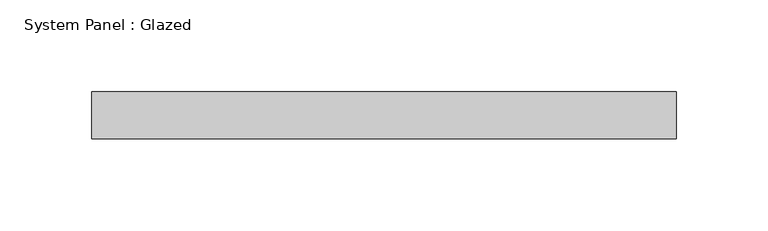
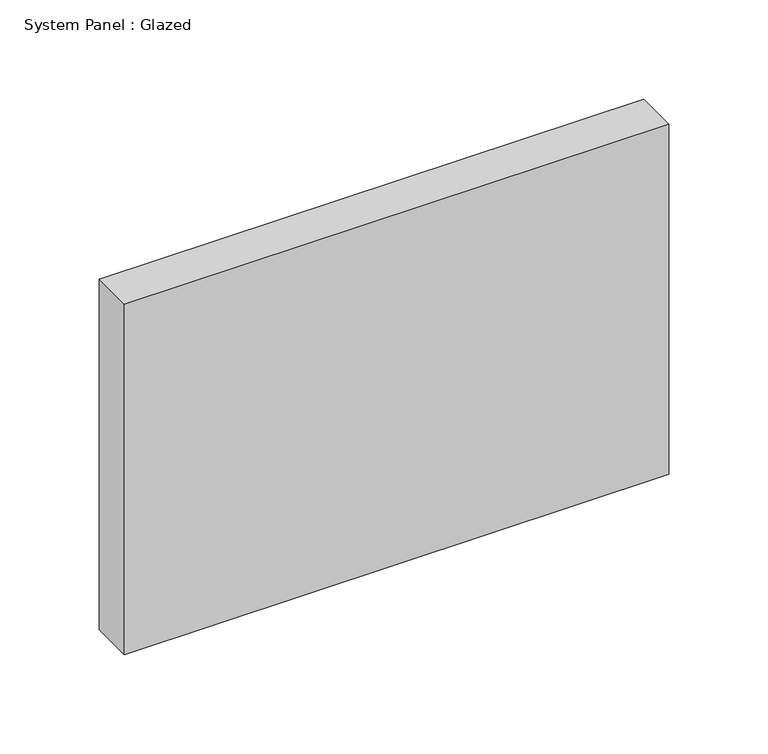
"""IFC4 building model written with IfcOpenShell, lengths in millimetres: plate geometry, System Panel : Glazed."""

from ifc_helpers import new_model, si_unit, origin, origin_with_axes, place, context, project, spatial, polyline, outline, extrude, source, transform, mapped, element, save


def system_panel_glazed_5633d65b(model_context):
    return source(origin(), model_context, "Body", "SweptSolid", [
        extrude(outline(polyline([(158.75, 19.05), (-158.75, 19.05), (-158.75, 44.45), (158.75, 44.45), (158.75, 19.05)])), origin_with_axes(), (0.0, 0.0, 1.0), 215.9),
    ])


if __name__ == "__main__":
    model = new_model("IFC4")
    model_context = context("Model", 3, world=origin())
    ifc_project = project(units=[si_unit("LENGTHUNIT", "METRE", prefix="MILLI")], contexts=[model_context])
    site = spatial("IfcSite", under=ifc_project)
    building = spatial("IfcBuilding", under=site)
    placement = place(None, origin())
    system_panel_glazed_shape = system_panel_glazed_5633d65b(model_context)
    element("IfcPlate", 1, ObjectType="System Panel : Glazed", at=placement, inside=building, context=model_context, shape_type="MappedRepresentation", body=[
        mapped(system_panel_glazed_shape, transform((0.0, 0.0, 0.0), x_axis=(1.0, 0.0, 0.0), y_axis=(0.0, 1.0, 0.0), z_axis=(0.0, 0.0, 1.0))),
    ])
    save(model, "model.ifc")

# Revit data of these elements
# Type "System Panel : Glazed"
#   Construction Type Id = "GSP4R"
#   Analytic Construction = "1/8 in Pilkington single glazing"
#   Visual Light Transmittance = 0.9
#   Solar Heat Gain Coefficient = 0.86
#   Heat Transfer Coefficient (U) = 1.18115 BTU/(h·ft²·°F)
#   Define Thermal Properties by = 1
# Element 1 (IfcPlate, "System Panel : Glazed")
#   Materials on its faces: "Glass"
# Materials
#   "Glass": class "Glass", colour RGB 0 128 192, transparency 0.75, Description = "Soda Lime Glass", Cost = 0
